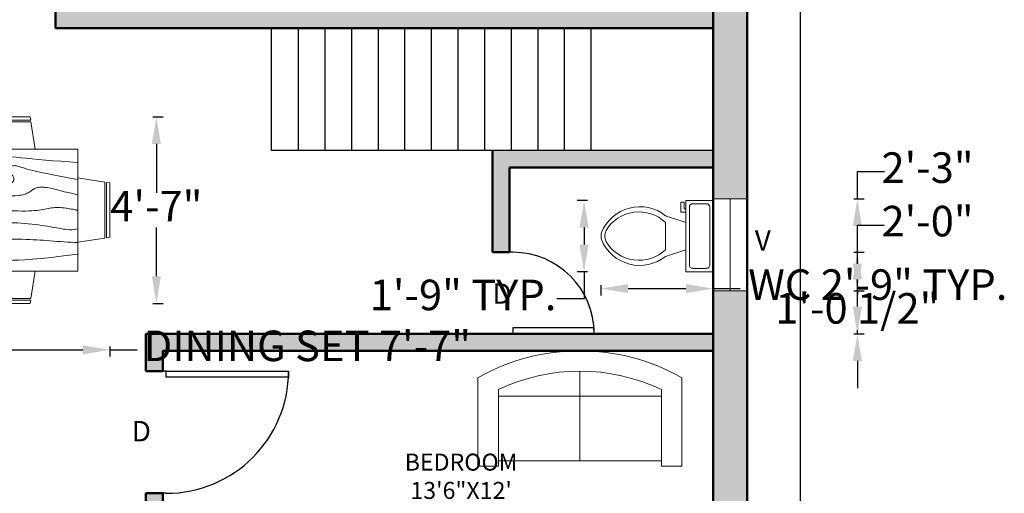
# Model space of a CAD drawing. Units: inches. Extents: x 2568 to 3190, y 746 to 1467.
# Tile 4 of 7: x 2900 to 3190, y 933 to 1073. Entities that reach past the tile are written whole.
import ezdxf

# ---------------------------------------------------------------- set-up
doc = ezdxf.new("R2010")
doc.units = ezdxf.units.IN
for name, color, linetype, lineweight in [('A-ANNO-DIMS', 2, 'Continuous', 18), ('A-ANNO-TEXT', 7, 'Continuous', 18), ('A-AREA-IDEN', 7, 'Continuous', 25), ('A-DOOR', 3, 'Continuous', 25), ('A-FLOR-FIXT', 9, 'Continuous', 20), ('A-FLOR-STRS', 7, 'Continuous', 25), ('A-FURN', 8, 'Continuous', 18), ('A-GLAZ', 4, 'Continuous', 20), ('A-WALL', 7, 'Continuous', 50), ('A-WALL-PATT', 252, 'Continuous', 13)]:
    doc.layers.add(name, color=color, linetype=linetype, lineweight=lineweight)
doc.styles.get("Standard").update_dxf_attribs({"font": 'arial.ttf'})
doc.dimstyles.new('ISO-25', dxfattribs={"dimtxt": 9, "dimasz": 8, "dimexe": 2, "dimexo": 1, "dimtad": 0, "dimtih": 1, "dimtoh": 1, "dimdec": 1, "dimlunit": 3, "dimtxsty": 'Standard', "dimcen": 2.5, "dimclrd": 1, "dimclre": 3, "dimclrt": 6, "dimadec": 0, "dimazin": 0, "dimtfac": 1, "dimtdec": 1, "dimtmove": 0, "dimatfit": 3, "dimfxl": 1, "dimfxlon": 1, "dimarcsym": 0})

# ---------------------------------------------------------------- blocks, each defined once
blk = doc.blocks.new('*U7')
for p, q in [((0, 0), (0, -6)), ((36, 0), (36, -6))]:
    blk.add_line(p, q)
blk.add_lwpolyline([(0, 0), (0, 36), (1.75, 36), (1.75, 0)], close=True)
blk.add_arc((0, 0), 36, 0, 90)
blk = doc.blocks.new('*U2')
for p, q in [((-24, 0), (-24, -6)), ((0, 0), (0, -6))]:
    blk.add_line(p, q)
blk.add_lwpolyline([(0, 0), (0, 24), (-1.75, 24), (-1.75, 0)], close=True)
blk.add_arc((0, 0), 24, 90, 180)
blk = doc.blocks.new('Dining Set - 36 x 72 in.')
for p, q in [((-22, 27.5), (-22.1562, 26.50042)), ((-5.8416, 26.5), (-22.1534, 26.5)), ((-22, 27.5), (-6, 27.5)), ((-5.8437, 26.49966), (-6, 27.5)), ((6, 27.5), (5.8438, 26.50042)), ((22.1584, 26.5), (5.8466, 26.5)), ((6, 27.5), (22, 27.5)), ((22.1563, 26.49966), (22, 27.5)), ((-22.2343, 26.00059), (-23.4847, 17.99762)), ((-22.2304, 26), (-5.7608, 26)), ((-4.5152, 17.99762), (-5.7655, 25.99926)), ((5.7657, 26.00059), (4.5153, 17.99762)), ((5.7696, 26), (22.2392, 26)), ((23.4848, 17.99762), (22.2345, 25.99926)), ((36, 18), (-36, 18)), ((-36, 18), (-36, -18)), ((36, -18), (36, 18)), ((-44.0006, 8.23428), (-35.9976, 9.48474)), ((44.0006, 8.23428), (35.9976, 9.48474)), ((-45.5, 8), (-44.5004, 8.15617)), ((-45.5, 8), (-45.5, -8)), ((-44.5, -8.15843), (-44.5, 8.15338)), ((-44, 8.23041), (-44, -8.23915)), ((44, 8.23041), (44, -8.23915)), ((44.5, -8.15843), (44.5, 8.15338)), ((45.5, 8), (44.5005, 8.15617)), ((45.5, 8), (45.5, -8)), ((-44.4997, -8.15631), (-45.5, -8)), ((-35.9976, -9.48476), (-43.9993, -8.2345)), ((35.9976, -9.48476), (43.9993, -8.2345)), ((44.4997, -8.15631), (45.5, -8)), ((-36, -18), (36, -18)), ((-22.2343, -26.0006), (-23.4847, -17.99762)), ((-4.5152, -17.99762), (-5.7655, -25.99928)), ((5.7657, -26.0006), (4.5153, -17.99762)), ((23.4848, -17.99762), (22.2345, -25.99928)), ((-22.2304, -26), (-5.7608, -26)), ((5.7696, -26), (22.2392, -26)), ((-22, -27.5), (-22.1562, -26.50044)), ((-5.8416, -26.5), (-22.1534, -26.5)), ((-22, -27.5), (-6, -27.5)), ((-5.8437, -26.49967), (-6, -27.5)), ((6, -27.5), (5.8438, -26.50044)), ((22.1584, -26.5), (5.8466, -26.5)), ((6, -27.5), (22, -27.5)), ((22.1563, -26.49967), (22, -27.5))]:
    blk.add_line(p, q)
for points in [[(-36, 15), (-31.1772, 14.97754), (-26.8079, 14.91406), (-22.8538, 14.81543), (-19.276, 14.6875), (-16.0362, 14.53613), (-13.0957, 14.36718), (-10.4159, 14.18652), (-7.9583, 14), (-5.6904, 13.81315), (-3.6035, 13.63021), (-1.6954, 13.45508), (0.0365, 13.29166), (1.5945, 13.14388), (2.9811, 13.01562), (4.1988, 12.9108), (5.25, 12.83333), (6.1393, 12.78613), (6.8802, 12.76823), (7.4883, 12.77767), (7.9792, 12.8125), (8.3685, 12.87077), (8.6719, 12.95052), (8.9049, 13.0498), (9.0833, 13.16666), (9.2205, 13.29899), (9.3216, 13.44401), (9.3895, 13.59879), (9.4271, 13.76041), (9.4373, 13.92594), (9.4232, 14.09245), (9.3875, 14.257), (9.3333, 14.41666), (9.2638, 14.56917), (9.1836, 14.71484), (9.0975, 14.85465), (9.0104, 14.98958), (8.9272, 15.1206), (8.8529, 15.2487), (8.7922, 15.37483), (8.75, 15.5), (8.7305, 15.62467), (8.7344, 15.74739), (8.7617, 15.86621), (8.8125, 15.97916), (8.8867, 16.08431), (8.9844, 16.17968), (9.1055, 16.26334), (9.25, 16.33333), (9.4189, 16.38802), (9.6172, 16.42708), (9.8506, 16.45052), (10.125, 16.45833), (10.4463, 16.45052), (10.8203, 16.42708), (11.2529, 16.38802), (11.75, 16.33333), (12.3184, 16.26318), (12.9694, 16.17838), (13.7151, 16.07991), (14.5677, 15.96875), (15.5395, 15.84586), (16.6426, 15.71224), (17.8893, 15.56884), (19.2917, 15.41666), (20.859, 15.25667), (22.5879, 15.08984), (24.4721, 14.91715), (26.5052, 14.73958), (28.6809, 14.5581), (30.9929, 14.3737), (33.4347, 14.18733), (36, 14)], [(-36, 10), (-28.9766, 10.14274), (-23.1725, 10.20442), (-18.4241, 10.19775), (-14.5677, 10.13541), (-11.4399, 10.03011), (-8.877, 9.89453), (-6.7154, 9.74137), (-4.7917, 9.58333), (-2.9698, 9.43082), (-1.2246, 9.28515), (0.4415, 9.14534), (2.026, 9.01041), (3.5266, 8.87939), (4.9408, 8.7513), (6.266, 8.62516), (7.5, 8.5), (8.6411, 8.37549), (9.6914, 8.2539), (10.6538, 8.13818), (11.5312, 8.03125), (12.3267, 7.93603), (13.043, 7.85547), (13.6831, 7.79248), (14.25, 7.75), (14.7471, 7.7303), (15.1797, 7.73307), (15.5537, 7.75732), (15.875, 7.80208), (16.1494, 7.86637), (16.3828, 7.94922), (16.5811, 8.04964), (16.75, 8.16666), (16.8944, 8.29915), (17.0143, 8.44531), (17.1089, 8.60319), (17.1771, 8.77083), (17.218, 8.94629), (17.2305, 9.1276), (17.2137, 9.31282), (17.1667, 9.5), (17.0895, 9.6875), (16.987, 9.875), (16.8649, 10.0625), (16.7292, 10.25), (16.5856, 10.4375), (16.4401, 10.625), (16.2985, 10.8125), (16.1667, 11), (16.05, 11.18733), (15.9518, 11.3737), (15.8752, 11.5581), (15.8229, 11.73958), (15.798, 11.91715), (15.8034, 12.08984), (15.842, 12.25667), (15.9167, 12.41666), (16.0295, 12.56836), (16.1784, 12.70833), (16.3605, 12.83268), (16.5729, 12.9375), (16.8127, 13.01888), (17.0768, 13.07291), (17.3625, 13.0957), (17.6667, 13.08333), (17.9894, 13.03312), (18.3418, 12.94726), (18.7382, 12.82918), (19.1927, 12.68229), (19.7195, 12.51001), (20.3327, 12.31575), (21.0465, 12.10294), (21.875, 11.875), (22.8357, 11.63354), (23.959, 11.37304), (25.2786, 11.08618), (26.8282, 10.76562), (28.6414, 10.40405), (30.752, 9.99414), (33.1936, 9.52856), (36, 9)], [(-36, 5.5), (-30.7157, 5.3348), (-26.069, 5.20963), (-21.9946, 5.11767), (-18.4271, 5.05208), (-15.3009, 5.00602), (-12.5508, 4.97265), (-10.1112, 4.94515), (-7.9167, 4.91666), (-5.909, 4.88167), (-4.0586, 4.83984), (-2.3429, 4.79215), (-0.7396, 4.73958), (0.7739, 4.6831), (2.22, 4.6237), (3.6213, 4.56233), (5, 4.5), (6.373, 4.43782), (7.7344, 4.3776), (9.0723, 4.32129), (10.375, 4.27083), (11.6309, 4.22819), (12.8281, 4.19531), (13.9551, 4.17415), (15, 4.16666), (15.954, 4.17448), (16.819, 4.19791), (17.6001, 4.23698), (18.3021, 4.29166), (18.9299, 4.36198), (19.4883, 4.44791), (19.9823, 4.54948), (20.4167, 4.66666), (20.7969, 4.79899), (21.1302, 4.94401), (21.4245, 5.09879), (21.6875, 5.26041), (21.9271, 5.42594), (22.1511, 5.59245), (22.3672, 5.757), (22.5834, 5.91666), (22.8065, 6.06868), (23.0404, 6.21093), (23.2879, 6.34147), (23.5521, 6.45833), (23.8358, 6.55957), (24.142, 6.64323), (24.4735, 6.70735), (24.8334, 6.75), (25.2235, 6.76969), (25.642, 6.76692), (26.0858, 6.74267), (26.5521, 6.69791), (27.0379, 6.63362), (27.5404, 6.55078), (28.0565, 6.45036), (28.5834, 6.33333), (29.1242, 6.19987), (29.7071, 6.04687), (30.3661, 5.87044), (31.1354, 5.66666), (32.0493, 5.43164), (33.142, 5.16146), (34.4475, 4.85221), (36, 4.5)], [(-36, -1), (-30.7915, -0.6591), (-26.0195, -0.38216), (-21.6519, -0.16284), (-17.6563, 0.00521), (-14.0005, 0.12833), (-10.6523, 0.21289), (-7.5796, 0.26522), (-4.75, 0.29166), (-2.134, 0.29793), (0.2878, 0.28711), (2.5317, 0.26163), (4.6146, 0.22396), (6.5529, 0.17651), (8.3633, 0.12174), (10.0623, 0.06209), (11.6667, 0), (13.1899, -0.06201), (14.6341, -0.1211), (15.9982, -0.17432), (17.2813, -0.21875), (18.4823, -0.25147), (19.6003, -0.26953), (20.6343, -0.27002), (21.5834, -0.25), (22.4481, -0.20768), (23.2357, -0.14584), (23.9549, -0.06836), (24.6146, 0.02083), (25.2235, 0.11784), (25.7904, 0.21875), (26.3241, 0.31966), (26.8334, 0.41666), (27.3265, 0.50618), (27.8099, 0.58593), (28.2894, 0.65397), (28.7709, 0.70833), (29.2601, 0.74707), (29.763, 0.76823), (30.2855, 0.76985), (30.8334, 0.75), (31.4088, 0.70784), (31.9994, 0.64713), (32.589, 0.57275), (33.1615, 0.48958), (33.7008, 0.4025), (34.1908, 0.3164), (34.6153, 0.23616), (34.9584, 0.16666), (35.2099, 0.11165), (35.3848, 0.07031), (35.504, 0.04069), (35.5886, 0.02083), (35.6594, 0.00879), (35.7377, 0.0026), (35.8442, 0.00032), (36, 0)], [(-36, -6.5), (-27.1843, -6.31267), (-20.084, -6.1263), (-14.469, -5.9419), (-10.1094, -5.76042), (-6.7752, -5.58285), (-4.2363, -5.41016), (-2.2629, -5.24333), (-0.625, -5.08334), (0.8708, -4.93099), (2.2715, -4.78646), (3.5872, -4.64974), (4.8281, -4.52084), (6.0046, -4.39974), (7.127, -4.28646), (8.2053, -4.18099), (9.25, -4.08334), (10.2705, -3.99382), (11.2734, -3.91407), (12.2647, -3.84603), (13.25, -3.79167), (14.2354, -3.75293), (15.2266, -3.73177), (16.2295, -3.73015), (17.25, -3.75), (18.2912, -3.79248), (19.3451, -3.85547), (20.4009, -3.93604), (21.4479, -4.03125), (22.4754, -4.13819), (23.4727, -4.25391), (24.4289, -4.37549), (25.3334, -4.5), (26.1785, -4.62492), (26.9694, -4.74935), (27.7145, -4.87281), (28.4219, -4.99479), (29.1, -5.11483), (29.7572, -5.23242), (30.4016, -5.34709), (31.0417, -5.45834), (31.6837, -5.56437), (32.3262, -5.65821), (32.9658, -5.73153), (33.599, -5.77604), (34.2224, -5.78345), (34.8327, -5.74545), (35.4264, -5.65373), (36, -5.5)], [(-36, -10), (-26.4022, -9.81299), (-18.4675, -9.62891), (-11.9839, -9.45069), (-6.7396, -9.28125), (-2.5226, -9.12354), (0.8789, -8.98047), (3.6769, -8.85498), (6.0833, -8.75), (8.2767, -8.66765), (10.3021, -8.60677), (12.1712, -8.56543), (13.8958, -8.54167), (15.4876, -8.53353), (16.9583, -8.53907), (18.3197, -8.55632), (19.5834, -8.58334), (20.7616, -8.61841), (21.8685, -8.66081), (22.9188, -8.71004), (23.9271, -8.76563), (24.9081, -8.82707), (25.8763, -8.89388), (26.8465, -8.96558), (27.8334, -9.04167), (28.8474, -9.12118), (29.8828, -9.20117), (30.93, -9.27824), (31.9792, -9.34896), (33.0205, -9.40991), (34.0443, -9.45768), (35.0407, -9.48885), (36, -9.5)], [(-36, -14.5), (-30.0881, -14.33513), (-25.0332, -14.21224), (-20.7312, -14.12647), (-17.0781, -14.07292), (-13.97, -14.04671), (-11.3027, -14.04297), (-8.9724, -14.05681), (-6.875, -14.08334), (-4.9224, -14.11833), (-3.0905, -14.16016), (-1.3709, -14.20785), (0.2448, -14.26042), (1.7647, -14.3169), (3.1973, -14.3763), (4.5507, -14.43767), (5.8333, -14.5), (7.0554, -14.5621), (8.235, -14.62175), (9.3922, -14.67652), (10.5469, -14.72396), (11.7192, -14.76164), (12.929, -14.78711), (14.1965, -14.79794), (15.5417, -14.79167), (16.9933, -14.76424), (18.6152, -14.70508), (20.4804, -14.60197), (22.6615, -14.44271), (25.2312, -14.21509), (28.2624, -13.9069), (31.8277, -13.50594), (36, -13)]]:
    blk.add_lwpolyline(points)
blk = doc.blocks.new('Toilet - top')
for p, q in [((9.5, -6), (9.5, -2)), ((-10, -8.5), (-8, -8.5)), ((-10, -9.5), (-10, -8.5)), ((-8, -8.5), (-8, -8)), ((-7, -8), (-7, -9.5)), ((-4, -8), (-6, -14)), ((4, -8), (6, -14)), ((-7, -9.5), (-10, -9.5)), ((4, -14), (-4, -14))]:
    blk.add_line(p, q)
blk.add_lwpolyline([(10.5, -8), (10.5, 0), (-10.5, 0), (-10.5, -8)], close=True)
for points in [[(-9.5, -2), (-9.5, -6)], [(8.5, -1), (-8.5, -1)], [(-8.5, -7), (8.5, -7)]]:
    blk.add_lwpolyline(points)
for centre, radius, start, end in [((-8.62, -1.88), 0.884, 81.8699, 188.1301), ((8.62, -1.88), 0.884, 351.8699, 98.1301), ((-8.62, -6.12), 0.884, 171.8699, 278.1301), ((8.62, -6.12), 0.884, 261.8699, 8.1301), ((3.52, -21.58), 12.17, 141.4691, 247.9714), ((4.2, -21.82), 11.33, 136.3677, 238.9468), ((-3.52, -21.58), 12.17, 292.0284, 38.5307), ((-4.2, -21.82), 11.33, 301.053, 43.6321), ((0, -27.88), 4, 245.7318, 294.2682), ((0, -29), 4, 254.8605, 285.1395)]:
    blk.add_arc(centre, radius, start, end)
blk = doc.blocks.new('*D14')
at = {"layer": 'A-ANNO-DIMS', "color": 0, "lineweight": -2, "transparency": 16777216}
for p, q in [((3129.28, 1421.35), (3132.28, 1421.35)), ((3130.28, 1413.35), (3130.28, 1126.57)), ((3130.28, 829.35), (3130.28, 1116.13)), ((3129.28, 821.35), (3132.28, 821.35))]:
    blk.add_line(p, q, dxfattribs=at)
at = {"layer": 'A-ANNO-DIMS', "color": 0, "transparency": 16777216}
for points in [[(3128.95, 1413.35), (3131.61, 1413.35), (3130.28, 1421.35)], [(3128.95, 829.35), (3131.61, 829.35), (3130.28, 821.35)]]:
    blk.add_solid(points, dxfattribs=at)
at = {"layer": 'Defpoints', "color": 0, "transparency": 16777216}
for p in [(3114.52, 1421.35), (3114.52, 821.35), (3130.28, 821.35)]:
    blk.add_point(p, dxfattribs=at)
at = {"layer": 'A-ANNO-DIMS', "color": 0, "transparency": 16777216, "insert": (3130.28, 1121.35), "char_height": 9, "attachment_point": 5}
blk.add_mtext("50'", dxfattribs=at)
blk = doc.blocks.new('Sofa - Roundback Loveseat 5 ft.')
for p, q in [((0, -32.44198), (0, -5.99998)), ((-24, -33.99998), (-24, -11.46958)), ((24.00004, -33.99998), (24.00004, -11.46958)), ((-23.9998, -13.38178), (23.99986, -13.38178)), ((-24, -32.44198), (24.00004, -32.44198))]:
    blk.add_line(p, q)
for points in [[(-24, -33.99998), (-30, -33.99998), (-30, -7.99998)], [(30.00004, -7.99998), (30.00004, -33.99998), (24.00004, -33.99998)]]:
    blk.add_lwpolyline(points)
for centre, radius, start, end in [((0, -60.24998), 60.24998, 60.13715, 119.8628), ((0, -61.38438), 55.38444, 64.32083, 115.6792)]:
    blk.add_arc(centre, radius, start, end)
blk = doc.blocks.new('*D27')
at = {"layer": 'A-ANNO-DIMS', "color": 3, "lineweight": -2, "transparency": 16777216}
for p, q in [((3071.48, 994.65), (3071.48, 991.65)), ((3104.52, 994.65), (3104.52, 991.65))]:
    blk.add_line(p, q, dxfattribs=at)
at = {"layer": 'A-ANNO-DIMS', "color": 1, "lineweight": -2, "transparency": 16777216}
for p, q in [((3079.48, 993.65), (3096.52, 993.65)), ((3104.52, 993.65), (3112.52, 993.65))]:
    blk.add_line(p, q, dxfattribs=at)
at = {"layer": 'A-ANNO-DIMS', "color": 1, "transparency": 16777216}
for points in [[(3079.48, 994.99), (3079.48, 992.32), (3071.48, 993.65)], [(3096.52, 994.99), (3096.52, 992.32), (3104.52, 993.65)]]:
    blk.add_solid(points, dxfattribs=at)
at = {"layer": 'Defpoints', "color": 0, "transparency": 16777216}
for p in [(3071.48, 998.61), (3104.52, 998.61), (3104.52, 993.65)]:
    blk.add_point(p, dxfattribs=at)
at = {"layer": 'A-ANNO-DIMS', "color": 6, "transparency": 16777216, "insert": (3152.98, 993.65), "char_height": 9, "attachment_point": 5}
blk.add_mtext('WC 2\'-9" TYP.', dxfattribs=at)
blk = doc.blocks.new('*D28')
at = {"layer": 'A-ANNO-DIMS', "color": 3, "lineweight": -2, "transparency": 16777216}
for p, q in [((3067.52, 1019.61), (3064.52, 1019.61)), ((3067.52, 998.61), (3064.52, 998.61))]:
    blk.add_line(p, q, dxfattribs=at)
at = {"layer": 'A-ANNO-DIMS', "color": 1, "lineweight": -2, "transparency": 16777216}
for p, q in [((3066.52, 1011.61), (3066.52, 1006.61)), ((3066.52, 998.61), (3066.52, 990.61)), ((3066.52, 990.61), (3058.52, 990.61))]:
    blk.add_line(p, q, dxfattribs=at)
at = {"layer": 'A-ANNO-DIMS', "color": 1, "transparency": 16777216}
for points in [[(3065.19, 1011.61), (3067.85, 1011.61), (3066.52, 1019.61)], [(3065.19, 1006.61), (3067.85, 1006.61), (3066.52, 998.61)]]:
    blk.add_solid(points, dxfattribs=at)
at = {"layer": 'Defpoints', "color": 0, "transparency": 16777216}
for p in [(3071.48, 1019.61), (3066.52, 998.61), (3071.48, 998.61)]:
    blk.add_point(p, dxfattribs=at)
at = {"layer": 'A-ANNO-DIMS', "color": 6, "transparency": 16777216, "insert": (3030.89, 990.61), "char_height": 9, "attachment_point": 5}
blk.add_mtext('1\'-9" TYP.', dxfattribs=at)
blk = doc.blocks.new('*D37')
at = {"layer": 'A-ANNO-DIMS', "color": 3, "lineweight": -2, "transparency": 16777216}
for p, q in [((2835.95, 976.61), (2835.95, 973.61)), ((2926.95, 976.61), (2926.95, 973.61))]:
    blk.add_line(p, q, dxfattribs=at)
at = {"layer": 'A-ANNO-DIMS', "color": 1, "lineweight": -2, "transparency": 16777216}
for p, q in [((2843.95, 975.61), (2918.95, 975.61)), ((2926.95, 975.61), (2934.95, 975.61))]:
    blk.add_line(p, q, dxfattribs=at)
at = {"layer": 'A-ANNO-DIMS', "color": 1, "transparency": 16777216}
for points in [[(2843.95, 976.94), (2843.95, 974.27), (2835.95, 975.61)], [(2918.95, 976.94), (2918.95, 974.27), (2926.95, 975.61)]]:
    blk.add_solid(points, dxfattribs=at)
at = {"layer": 'Defpoints', "color": 0, "transparency": 16777216}
for p in [(2835.95, 989.26), (2926.95, 989.26), (2926.95, 975.61)]:
    blk.add_point(p, dxfattribs=at)
at = {"layer": 'A-ANNO-DIMS', "color": 6, "transparency": 16777216, "insert": (2985.04, 975.61), "char_height": 9, "attachment_point": 5}
blk.add_mtext('DINING SET 7\'-7"', dxfattribs=at)
blk = doc.blocks.new('*D38')
at = {"layer": 'A-ANNO-DIMS', "color": 3, "lineweight": -2, "transparency": 16777216}
for p, q in [((2939.6, 1044.26), (2942.6, 1044.26)), ((2939.6, 989.26), (2942.6, 989.26))]:
    blk.add_line(p, q, dxfattribs=at)
at = {"layer": 'A-ANNO-DIMS', "color": 1, "lineweight": -2, "transparency": 16777216}
for p, q in [((2940.6, 1036.26), (2940.6, 1021.88)), ((2940.6, 997.26), (2940.6, 1011.63))]:
    blk.add_line(p, q, dxfattribs=at)
at = {"layer": 'A-ANNO-DIMS', "color": 1, "transparency": 16777216}
for points in [[(2939.27, 1036.26), (2941.94, 1036.26), (2940.6, 1044.26)], [(2939.27, 997.26), (2941.94, 997.26), (2940.6, 989.26)]]:
    blk.add_solid(points, dxfattribs=at)
at = {"layer": 'Defpoints', "color": 0, "transparency": 16777216}
for p in [(2926.95, 1044.26), (2940.6, 1044.26), (2926.95, 989.26)]:
    blk.add_point(p, dxfattribs=at)
at = {"layer": 'A-ANNO-DIMS', "color": 6, "transparency": 16777216, "insert": (2940.6, 1016.76), "char_height": 9, "attachment_point": 5}
blk.add_mtext('4\'-7"', dxfattribs=at)
blk = doc.blocks.new('*D43')
at = {"layer": 'A-ANNO-DIMS', "color": 1, "lineweight": -2, "transparency": 16777216}
for p, q in [((2934.52, 759.85), (2926.52, 759.85)), ((2942.52, 759.85), (2946.11, 759.85)), ((2996.2, 759.85), (2992.62, 759.85)), ((3004.2, 759.85), (3012.2, 759.85))]:
    blk.add_line(p, q, dxfattribs=at)
at = {"layer": 'A-ANNO-DIMS', "color": 3, "lineweight": -2, "transparency": 16777216}
for p, q in [((2942.52, 760.85), (2942.52, 757.85)), ((2996.2, 760.85), (2996.2, 757.85))]:
    blk.add_line(p, q, dxfattribs=at)
at = {"layer": 'A-ANNO-DIMS', "color": 1, "transparency": 16777216}
for points in [[(2934.52, 761.18), (2934.52, 758.51), (2942.52, 759.85)], [(3004.2, 761.18), (3004.2, 758.51), (2996.2, 759.85)]]:
    blk.add_solid(points, dxfattribs=at)
at = {"layer": 'Defpoints', "color": 0, "transparency": 16777216}
for p in [(2942.52, 1411.35), (2996.2, 1411.35), (2996.2, 759.85)]:
    blk.add_point(p, dxfattribs=at)
at = {"layer": 'A-ANNO-DIMS', "color": 6, "transparency": 16777216, "insert": (2969.36, 759.85), "char_height": 9, "attachment_point": 5}
blk.add_mtext('4\'-5 1/2"', dxfattribs=at)
blk = doc.blocks.new('*D44')
at = {"layer": 'A-ANNO-DIMS', "color": 1, "lineweight": -2, "transparency": 16777216}
for p, q in [((2988.2, 759.85), (2980.2, 759.85)), ((2996.2, 759.85), (3001.17, 759.85)), ((3052.64, 759.85), (3047.67, 759.85)), ((3060.64, 759.85), (3068.64, 759.85))]:
    blk.add_line(p, q, dxfattribs=at)
at = {"layer": 'A-ANNO-DIMS', "color": 3, "lineweight": -2, "transparency": 16777216}
for p, q in [((2996.2, 760.85), (2996.2, 757.85)), ((3052.64, 760.85), (3052.64, 757.85))]:
    blk.add_line(p, q, dxfattribs=at)
at = {"layer": 'A-ANNO-DIMS', "color": 1, "transparency": 16777216}
for points in [[(2988.2, 761.18), (2988.2, 758.51), (2996.2, 759.85)], [(3060.64, 761.18), (3060.64, 758.51), (3052.64, 759.85)]]:
    blk.add_solid(points, dxfattribs=at)
at = {"layer": 'Defpoints', "color": 0, "transparency": 16777216}
for p in [(2996.2, 1411.35), (3052.64, 1411.35), (3052.64, 759.85)]:
    blk.add_point(p, dxfattribs=at)
at = {"layer": 'A-ANNO-DIMS', "color": 6, "transparency": 16777216, "insert": (3024.42, 759.85), "char_height": 9, "attachment_point": 5}
blk.add_mtext('4\'-8 1/2"', dxfattribs=at)
blk = doc.blocks.new('*D50')
at = {"layer": 'A-ANNO-DIMS', "color": 3, "lineweight": -2, "transparency": 16777216}
for p, q in [((2846.86, 1452.8), (2846.86, 1455.8)), ((2902.21, 1452.8), (2902.21, 1455.8))]:
    blk.add_line(p, q, dxfattribs=at)
at = {"layer": 'A-ANNO-DIMS', "color": 1, "lineweight": -2, "transparency": 16777216}
for p, q in [((2838.86, 1453.8), (2830.86, 1453.8)), ((2846.86, 1453.8), (2851.29, 1453.8)), ((2902.21, 1453.8), (2897.79, 1453.8)), ((2910.21, 1453.8), (2918.21, 1453.8))]:
    blk.add_line(p, q, dxfattribs=at)
at = {"layer": 'A-ANNO-DIMS', "color": 1, "transparency": 16777216}
for points in [[(2838.86, 1455.13), (2838.86, 1452.47), (2846.86, 1453.8)], [(2910.21, 1455.13), (2910.21, 1452.47), (2902.21, 1453.8)]]:
    blk.add_solid(points, dxfattribs=at)
at = {"layer": 'Defpoints', "color": 0, "transparency": 16777216}
for p in [(2902.21, 1453.8), (2846.86, 831.35), (2902.21, 831.35)]:
    blk.add_point(p, dxfattribs=at)
at = {"layer": 'A-ANNO-DIMS', "color": 6, "transparency": 16777216, "insert": (2874.54, 1453.8), "char_height": 9, "attachment_point": 5}
blk.add_mtext('4\'-7 1/2"', dxfattribs=at)
blk = doc.blocks.new('*D56')
at = {"layer": 'A-ANNO-DIMS', "color": 3, "lineweight": -2, "transparency": 16777216}
for p, q in [((2603.07, 1070.35), (2600.07, 1070.35)), ((2603.07, 1034.35), (2600.07, 1034.35))]:
    blk.add_line(p, q, dxfattribs=at)
at = {"layer": 'A-ANNO-DIMS', "color": 1, "lineweight": -2, "transparency": 16777216}
for p, q in [((2602.07, 1062.35), (2602.07, 1057.57)), ((2602.07, 1042.35), (2602.07, 1047.13))]:
    blk.add_line(p, q, dxfattribs=at)
at = {"layer": 'A-ANNO-DIMS', "color": 1, "transparency": 16777216}
for points in [[(2600.74, 1062.35), (2603.41, 1062.35), (2602.07, 1070.35)], [(2600.74, 1042.35), (2603.41, 1042.35), (2602.07, 1034.35)]]:
    blk.add_solid(points, dxfattribs=at)
at = {"layer": 'Defpoints', "color": 0, "transparency": 16777216}
for p in [(2602.07, 1070.35), (2974.52, 1070.35), (2974.52, 1034.35)]:
    blk.add_point(p, dxfattribs=at)
at = {"layer": 'A-ANNO-DIMS', "color": 6, "transparency": 16777216, "insert": (2602.07, 1052.35), "char_height": 9, "attachment_point": 5}
blk.add_mtext('3\'-0"', dxfattribs=at)
blk = doc.blocks.new('*D57')
at = {"layer": 'A-ANNO-DIMS', "color": 3, "lineweight": -2, "transparency": 16777216}
for p, q in [((2974.52, 1452.8), (2974.52, 1455.8)), ((3104.52, 1452.8), (3104.52, 1455.8))]:
    blk.add_line(p, q, dxfattribs=at)
at = {"layer": 'A-ANNO-DIMS', "color": 1, "lineweight": -2, "transparency": 16777216}
for p, q in [((2982.52, 1453.8), (3020.37, 1453.8)), ((3096.52, 1453.8), (3058.68, 1453.8))]:
    blk.add_line(p, q, dxfattribs=at)
at = {"layer": 'A-ANNO-DIMS', "color": 1, "transparency": 16777216}
for points in [[(2982.52, 1455.13), (2982.52, 1452.47), (2974.52, 1453.8)], [(3096.52, 1455.13), (3096.52, 1452.47), (3104.52, 1453.8)]]:
    blk.add_solid(points, dxfattribs=at)
at = {"layer": 'Defpoints', "color": 0, "transparency": 16777216}
for p in [(3104.52, 1453.8), (2974.52, 1070.35), (3104.52, 1070.35)]:
    blk.add_point(p, dxfattribs=at)
at = {"layer": 'A-ANNO-DIMS', "color": 6, "transparency": 16777216, "insert": (3039.52, 1453.8), "char_height": 9, "attachment_point": 5}
blk.add_mtext('10\'-10"', dxfattribs=at)
blk = doc.blocks.new('*D58')
at = {"layer": 'A-ANNO-DIMS', "color": 3, "lineweight": -2, "transparency": 16777216}
for p, q in [((2603.07, 1029.35), (2600.07, 1029.35)), ((2603.07, 980.35), (2600.07, 980.35))]:
    blk.add_line(p, q, dxfattribs=at)
at = {"layer": 'A-ANNO-DIMS', "color": 1, "lineweight": -2, "transparency": 16777216}
for p, q in [((2602.07, 1021.35), (2602.07, 1009.99)), ((2602.07, 988.35), (2602.07, 999.71))]:
    blk.add_line(p, q, dxfattribs=at)
at = {"layer": 'A-ANNO-DIMS', "color": 1, "transparency": 16777216}
for points in [[(2600.74, 1021.35), (2603.41, 1021.35), (2602.07, 1029.35)], [(2600.74, 988.35), (2603.41, 988.35), (2602.07, 980.35)]]:
    blk.add_solid(points, dxfattribs=at)
at = {"layer": 'Defpoints', "color": 0, "transparency": 16777216}
for p in [(3044.52, 1029.35), (2602.07, 980.35), (3043.77, 980.35)]:
    blk.add_point(p, dxfattribs=at)
at = {"layer": 'A-ANNO-DIMS', "color": 6, "transparency": 16777216, "insert": (2602.07, 1004.85), "char_height": 9, "attachment_point": 5}
blk.add_mtext('4\'-1"', dxfattribs=at)
blk = doc.blocks.new('*D59')
at = {"layer": 'A-ANNO-DIMS', "color": 3, "lineweight": -2, "transparency": 16777216}
for p, q in [((3044.52, 760.85), (3044.52, 757.85)), ((3104.52, 760.85), (3104.52, 757.85))]:
    blk.add_line(p, q, dxfattribs=at)
at = {"layer": 'A-ANNO-DIMS', "color": 1, "lineweight": -2, "transparency": 16777216}
for p, q in [((3052.52, 759.85), (3061.94, 759.85)), ((3096.52, 759.85), (3087.11, 759.85))]:
    blk.add_line(p, q, dxfattribs=at)
at = {"layer": 'A-ANNO-DIMS', "color": 1, "transparency": 16777216}
for points in [[(3052.52, 761.18), (3052.52, 758.51), (3044.52, 759.85)], [(3096.52, 761.18), (3096.52, 758.51), (3104.52, 759.85)]]:
    blk.add_solid(points, dxfattribs=at)
at = {"layer": 'Defpoints', "color": 0, "transparency": 16777216}
for p in [(3044.52, 1029.35), (3104.52, 1029.35), (3104.52, 759.85)]:
    blk.add_point(p, dxfattribs=at)
at = {"layer": 'A-ANNO-DIMS', "color": 6, "transparency": 16777216, "insert": (3074.52, 759.85), "char_height": 9, "attachment_point": 5}
blk.add_mtext('5\'-0"', dxfattribs=at)
blk = doc.blocks.new('*D60')
at = {"layer": 'A-ANNO-DIMS', "color": 1, "lineweight": -2, "transparency": 16777216}
for p, q in [((2966.52, 759.85), (2958.52, 759.85)), ((2974.52, 759.85), (2982.36, 759.85)), ((2990.36, 759.85), (2998.36, 759.85))]:
    blk.add_line(p, q, dxfattribs=at)
at = {"layer": 'A-ANNO-DIMS', "color": 3, "lineweight": -2, "transparency": 16777216}
for p, q in [((2974.52, 760.85), (2974.52, 757.85)), ((2982.36, 760.85), (2982.36, 757.85))]:
    blk.add_line(p, q, dxfattribs=at)
at = {"layer": 'A-ANNO-DIMS', "color": 1, "transparency": 16777216}
for points in [[(2966.52, 761.18), (2966.52, 758.51), (2974.52, 759.85)], [(2990.36, 761.18), (2990.36, 758.51), (2982.36, 759.85)]]:
    blk.add_solid(points, dxfattribs=at)
at = {"layer": 'Defpoints', "color": 0, "transparency": 16777216}
for p in [(2974.52, 1034.35), (2982.36, 1034.35), (2982.36, 759.85)]:
    blk.add_point(p, dxfattribs=at)
at = {"layer": 'A-ANNO-DIMS', "color": 6, "transparency": 16777216, "insert": (3010.94, 759.85), "char_height": 9, "attachment_point": 5}
blk.add_mtext('0\'-8"', dxfattribs=at)
blk = doc.blocks.new('*D61')
at = {"layer": 'A-ANNO-DIMS', "color": 3, "lineweight": -2, "transparency": 16777216}
for p, q in [((3068.52, 1452.8), (3068.52, 1455.8)), ((3104.52, 1452.8), (3104.52, 1455.8))]:
    blk.add_line(p, q, dxfattribs=at)
at = {"layer": 'A-ANNO-DIMS', "color": 1, "lineweight": -2, "transparency": 16777216}
for p, q in [((3060.52, 1453.8), (3052.52, 1453.8)), ((3068.52, 1453.8), (3073.94, 1453.8)), ((3104.52, 1453.8), (3099.11, 1453.8)), ((3112.52, 1453.8), (3120.52, 1453.8))]:
    blk.add_line(p, q, dxfattribs=at)
at = {"layer": 'A-ANNO-DIMS', "color": 1, "transparency": 16777216}
for points in [[(3060.52, 1455.13), (3060.52, 1452.47), (3068.52, 1453.8)], [(3112.52, 1455.13), (3112.52, 1452.47), (3104.52, 1453.8)]]:
    blk.add_solid(points, dxfattribs=at)
at = {"layer": 'Defpoints', "color": 0, "transparency": 16777216}
for p in [(3104.52, 1453.8), (3068.52, 1034.35), (3104.52, 1034.35)]:
    blk.add_point(p, dxfattribs=at)
at = {"layer": 'A-ANNO-DIMS', "color": 6, "transparency": 16777216, "insert": (3086.52, 1453.8), "char_height": 9, "attachment_point": 5}
blk.add_mtext('3\'-0"', dxfattribs=at)
blk = doc.blocks.new('*D62')
at = {"layer": 'A-ANNO-DIMS', "color": 3, "lineweight": -2, "transparency": 16777216}
for p, q in [((2603.07, 1004.35), (2600.07, 1004.35)), ((2603.07, 980.35), (2600.07, 980.35))]:
    blk.add_line(p, q, dxfattribs=at)
at = {"layer": 'A-ANNO-DIMS', "color": 1, "lineweight": -2, "transparency": 16777216}
for p, q in [((2602.07, 996.35), (2602.07, 988.35)), ((2602.07, 980.35), (2602.07, 972.35)), ((2602.07, 972.35), (2594.07, 972.35))]:
    blk.add_line(p, q, dxfattribs=at)
at = {"layer": 'A-ANNO-DIMS', "color": 1, "transparency": 16777216}
for points in [[(2600.74, 996.35), (2603.41, 996.35), (2602.07, 1004.35)], [(2600.74, 988.35), (2603.41, 988.35), (2602.07, 980.35)]]:
    blk.add_solid(points, dxfattribs=at)
at = {"layer": 'Defpoints', "color": 0, "transparency": 16777216}
for p in [(3044.52, 1004.35), (2602.07, 980.35), (3043.77, 980.35)]:
    blk.add_point(p, dxfattribs=at)
at = {"layer": 'A-ANNO-DIMS', "color": 6, "transparency": 16777216, "insert": (2581.41, 972.35), "char_height": 9, "attachment_point": 5}
blk.add_mtext('2\'-0"', dxfattribs=at)
blk = doc.blocks.new('*D63')
at = {"layer": 'A-ANNO-DIMS', "color": 1, "lineweight": -2, "transparency": 16777216}
for p, q in [((3146.97, 1004.35), (3146.97, 1012.35)), ((3146.97, 1012.35), (3154.97, 1012.35)), ((3146.97, 988.35), (3146.97, 996.35))]:
    blk.add_line(p, q, dxfattribs=at)
at = {"layer": 'A-ANNO-DIMS', "color": 3, "lineweight": -2, "transparency": 16777216}
for p, q in [((3145.97, 1004.35), (3148.97, 1004.35)), ((3145.97, 980.35), (3148.97, 980.35))]:
    blk.add_line(p, q, dxfattribs=at)
at = {"layer": 'A-ANNO-DIMS', "color": 1, "transparency": 16777216}
for points in [[(3145.64, 996.35), (3148.31, 996.35), (3146.97, 1004.35)], [(3145.64, 988.35), (3148.31, 988.35), (3146.97, 980.35)]]:
    blk.add_solid(points, dxfattribs=at)
at = {"layer": 'Defpoints', "color": 0, "transparency": 16777216}
for p in [(2806.52, 1004.35), (3146.97, 1004.35), (2806.52, 980.35)]:
    blk.add_point(p, dxfattribs=at)
at = {"layer": 'A-ANNO-DIMS', "color": 6, "transparency": 16777216, "insert": (3167.64, 1012.35), "char_height": 9, "attachment_point": 5}
blk.add_mtext('2\'-0"', dxfattribs=at)
blk = doc.blocks.new('*D72')
at = {"layer": 'A-ANNO-DIMS', "color": 1, "lineweight": -2, "transparency": 16777216}
for p, q in [((3146.97, 1020.11), (3146.97, 1028.11)), ((3146.97, 1028.11), (3154.97, 1028.11)), ((3146.97, 1000.96), (3146.97, 1012.11))]:
    blk.add_line(p, q, dxfattribs=at)
at = {"layer": 'A-ANNO-DIMS', "color": 3, "lineweight": -2, "transparency": 16777216}
for p, q in [((3145.97, 1020.11), (3148.97, 1020.11)), ((3145.97, 992.96), (3148.97, 992.96))]:
    blk.add_line(p, q, dxfattribs=at)
at = {"layer": 'A-ANNO-DIMS', "color": 1, "transparency": 16777216}
for points in [[(3145.64, 1012.11), (3148.31, 1012.11), (3146.97, 1020.11)], [(3145.64, 1000.96), (3148.31, 1000.96), (3146.97, 992.96)]]:
    blk.add_solid(points, dxfattribs=at)
at = {"layer": 'Defpoints', "color": 0, "transparency": 16777216}
for p in [(3114.52, 1020.11), (3146.97, 1020.11), (3114.52, 992.96)]:
    blk.add_point(p, dxfattribs=at)
at = {"layer": 'A-ANNO-DIMS', "color": 6, "transparency": 16777216, "insert": (3167.64, 1028.11), "char_height": 9, "attachment_point": 5}
blk.add_mtext('2\'-3"', dxfattribs=at)
blk = doc.blocks.new('*D73')
at = {"layer": 'A-ANNO-DIMS', "color": 1, "lineweight": -2, "transparency": 16777216}
for p, q in [((3146.97, 1000.96), (3146.97, 1008.96)), ((3146.97, 992.96), (3146.97, 991.93)), ((3146.97, 980.35), (3146.97, 981.38)), ((3146.97, 972.35), (3146.97, 964.35))]:
    blk.add_line(p, q, dxfattribs=at)
at = {"layer": 'A-ANNO-DIMS', "color": 3, "lineweight": -2, "transparency": 16777216}
for p, q in [((3145.97, 992.96), (3148.97, 992.96)), ((3145.97, 980.35), (3148.97, 980.35))]:
    blk.add_line(p, q, dxfattribs=at)
at = {"layer": 'A-ANNO-DIMS', "color": 1, "transparency": 16777216}
for points in [[(3145.64, 1000.96), (3148.31, 1000.96), (3146.97, 992.96)], [(3145.64, 972.35), (3148.31, 972.35), (3146.97, 980.35)]]:
    blk.add_solid(points, dxfattribs=at)
at = {"layer": 'Defpoints', "color": 0, "transparency": 16777216}
for p in [(3104.52, 992.96), (3146.97, 992.96), (3104.52, 980.35)]:
    blk.add_point(p, dxfattribs=at)
at = {"layer": 'A-ANNO-DIMS', "color": 6, "transparency": 16777216, "insert": (3146.97, 986.66), "char_height": 9, "attachment_point": 5}
blk.add_mtext('1\'-0 1/2"', dxfattribs=at)
blk = doc.blocks.new('*D76')
at = {"layer": 'A-ANNO-DIMS', "color": 3, "lineweight": -2, "transparency": 16777216}
for p, q in [((3044.52, 760.85), (3044.52, 757.85)), ((3104.52, 760.85), (3104.52, 757.85))]:
    blk.add_line(p, q, dxfattribs=at)
at = {"layer": 'A-ANNO-DIMS', "color": 1, "lineweight": -2, "transparency": 16777216}
for p, q in [((3052.52, 759.85), (3061.94, 759.85)), ((3096.52, 759.85), (3087.11, 759.85))]:
    blk.add_line(p, q, dxfattribs=at)
at = {"layer": 'A-ANNO-DIMS', "color": 1, "transparency": 16777216}
for points in [[(3052.52, 761.18), (3052.52, 758.51), (3044.52, 759.85)], [(3096.52, 761.18), (3096.52, 758.51), (3104.52, 759.85)]]:
    blk.add_solid(points, dxfattribs=at)
at = {"layer": 'Defpoints', "color": 0, "transparency": 16777216}
for p in [(3044.52, 1202.35), (3104.52, 1202.35), (3104.52, 759.85)]:
    blk.add_point(p, dxfattribs=at)
at = {"layer": 'A-ANNO-DIMS', "color": 6, "transparency": 16777216, "insert": (3074.52, 759.85), "char_height": 9, "attachment_point": 5}
blk.add_mtext('5\'-0"', dxfattribs=at)

msp = doc.modelspace()

# ---------------------------------------------------------------- hatches: boundary and pattern name
at = {"layer": 'A-WALL-PATT'}
h = msp.add_hatch(color=256, dxfattribs=at)
h.dxf.hatch_style = 1
h.paths.add_polyline_path([(2709.74, 1411.35), (2709.74, 1421.35), (2634.52, 1421.35), (2634.52, 1371.08), (2644.52, 1371.08), (2644.52, 1411.35)])
h.paths.add_polyline_path([(2844.66, 1411.35), (2844.66, 1421.35), (2763.78, 1421.35), (2763.78, 1411.35)])
h.paths.add_polyline_path([(2996.2, 1411.35), (2996.2, 1421.35), (2897.43, 1421.35), (2897.43, 1411.35)])
h.paths.add_polyline_path([(3104.52, 1411.35), (3104.52, 1371.08), (3114.52, 1371.08), (3114.52, 1421.35), (3052.64, 1421.35), (3052.64, 1411.35)])
h.paths.add_polyline_path([(3114.52, 1316.62), (3104.52, 1316.62), (3104.52, 1248.37), (3114.52, 1248.37)])
h.paths.add_polyline_path([(3104.52, 1174.04), (3114.52, 1174.04), (3114.52, 1222.08), (3104.52, 1222.08)])
h.paths.add_polyline_path([(3104.52, 1020.11), (3114.52, 1020.11), (3114.52, 1113), (3104.52, 1113)])
h.paths.add_polyline_path([(3104.52, 920.42), (3114.52, 920.42), (3114.52, 992.96), (3104.52, 992.96)])
h.paths.add_polyline_path([(3114.52, 821.35), (3114.52, 865.93), (3104.52, 865.93), (3104.52, 831.35), (3055.78, 831.35), (3055.78, 821.35)])
h.paths.add_polyline_path([(2902.21, 831.35), (2902.21, 821.35), (2986.63, 821.35), (2986.63, 831.35)])
h.paths.add_polyline_path([(2634.52, 821.35), (2676.76, 821.35), (2676.76, 831.35), (2644.52, 831.35), (2644.52, 865.93), (2634.52, 865.93)])
h.paths.add_polyline_path([(2754.37, 821.35), (2846.86, 821.35), (2846.86, 831.35), (2754.37, 831.35)])
h.paths.add_polyline_path([(2644.52, 920.42), (2644.52, 1002.57), (2634.52, 1002.57), (2634.52, 920.42)])
h.paths.add_polyline_path([(2644.52, 1044.16), (2644.52, 1113), (2634.52, 1113), (2634.52, 1044.16)])
h.paths.add_polyline_path([(2644.52, 1248.37), (2644.52, 1316.62), (2634.52, 1316.62), (2634.52, 1248.37)])
h.paths.add_polyline_path([(2634.52, 1222.08), (2634.52, 1174.04), (2644.52, 1174.04), (2644.52, 1222.08)])
h = msp.add_hatch(color=256, dxfattribs=at)
h.dxf.hatch_style = 1
h.paths.add_polyline_path([(2811.52, 1411.35), (2806.52, 1411.35), (2806.52, 1303.35), (2811.52, 1303.35), (2811.52, 1310.35), (2850.52, 1310.35), (2850.52, 1315.35), (2811.52, 1315.35)])
h.paths.add_polyline_path([(2942.52, 1411.35), (2937.52, 1411.35), (2937.52, 1315.35), (2898.52, 1315.35), (2898.52, 1310.35), (2937.52, 1310.35), (2937.52, 1303.35), (2942.52, 1303.35)])
h.paths.add_polyline_path([(2811.52, 1267.35), (2704.52, 1267.35), (2704.52, 1261.35), (2704.52, 1237.35), (2704.52, 1202.35), (2644.52, 1202.35), (2644.52, 1197.35), (2806.52, 1197.35), (2806.52, 1191.38), (2811.52, 1191.38), (2811.52, 1202.35), (2793.52, 1202.35), (2793.52, 1232.35), (2788.52, 1232.35), (2788.52, 1202.35), (2709.52, 1202.35), (2709.52, 1262.35), (2788.52, 1262.35), (2788.52, 1256.35), (2793.52, 1256.35), (2793.52, 1262.35), (2811.52, 1262.35)])
h.paths.add_polyline_path([(2680.52, 1267.35), (2644.52, 1267.35), (2644.52, 1261.35), (2680.52, 1261.35)])
h.paths.add_polyline_path([(3044.52, 1267.35), (2937.52, 1267.35), (2937.52, 1262.35), (2955.52, 1262.35), (2955.52, 1256.35), (2960.52, 1256.35), (2960.52, 1262.35), (3039.52, 1262.35), (3039.52, 1202.35), (2960.52, 1202.35), (2960.52, 1232.35), (2955.52, 1232.35), (2955.52, 1202.35), (2937.52, 1202.35), (2937.52, 1191.38), (2942.52, 1191.38), (2942.52, 1197.35), (3104.52, 1197.35), (3104.52, 1202.35), (3044.52, 1202.35)])
h.paths.add_polyline_path([(3104.52, 1267.35), (3072.52, 1267.35), (3072.52, 1262.35), (3104.52, 1262.35)])
h.paths.add_polyline_path([(2838.1, 1075.35), (2811.52, 1075.35), (2811.52, 1155.35), (2806.52, 1155.35), (2806.52, 1075.35), (2644.52, 1075.35), (2644.52, 1070.35), (2806.52, 1070.35), (2811.52, 1070.35), (2838.1, 1070.35)])
h.paths.add_polyline_path([(3104.52, 1075.35), (2942.52, 1075.35), (2942.52, 1155.38), (2937.52, 1155.38), (2937.52, 1075.35), (2910.92, 1075.35), (2910.92, 1070.35), (2937.52, 1070.35), (3104.52, 1070.35)])
h.paths.add_polyline_path([(2811.52, 1038.35), (2806.52, 1038.35), (2806.52, 980.35), (2644.52, 980.35), (2644.52, 975.35), (2806.52, 975.35), (2806.52, 969.37), (2811.52, 969.37), (2811.52, 975.35)])
h.paths.add_polyline_path([(3104.52, 980.35), (2937.52, 980.35), (2937.52, 969.35), (2942.52, 969.35), (2942.52, 975.35), (3104.52, 975.35)])
h.paths.add_polyline_path([(3104.52, 1034.35), (3039.52, 1034.35), (3039.52, 1004.35), (3044.52, 1004.35), (3044.52, 1029.35), (3104.52, 1029.35)])
h.paths.add_polyline_path([(2942.52, 933.35), (2937.52, 933.35), (2937.52, 831.35), (2942.52, 831.35)])
h.paths.add_polyline_path([(2811.52, 933.37), (2806.52, 933.37), (2806.52, 831.35), (2811.52, 831.35)])

# ---------------------------------------------------------------- linework, layer by layer
at = {"layer": 'A-FLOR-STRS'}
for p, q in [((2974.52, 1034.35), (2974.52, 1070.35)), ((2982.36, 1070.35), (2982.36, 1034.35)), ((2990.19, 1070.35), (2990.19, 1034.35)), ((2998.02, 1070.35), (2998.02, 1034.35)), ((3005.86, 1070.35), (3005.86, 1034.35)), ((3013.69, 1070.35), (3013.69, 1034.35)), ((3021.52, 1070.35), (3021.52, 1034.35)), ((3029.36, 1070.35), (3029.36, 1034.35)), ((3037.19, 1070.35), (3037.19, 1034.35)), ((3045.02, 1070.35), (3045.02, 1034.35)), ((3052.86, 1070.35), (3052.86, 1034.35)), ((3060.69, 1070.35), (3060.69, 1034.35)), ((3068.52, 1070.35), (3068.52, 1034.35)), ((3104.52, 1034.35), (2974.52, 1034.35))]:
    msp.add_line(p, q, dxfattribs=at)
at = {"layer": 'A-GLAZ'}
for p, q in [((3104.52, 1020.11), (3114.52, 1020.11)), ((3109.52, 992.96), (3109.52, 1020.11)), ((3104.52, 992.96), (3114.52, 992.96))]:
    msp.add_line(p, q, dxfattribs=at)
at = {"layer": 'A-WALL'}
for p, q in [((3114.52, 821.35), (3114.52, 1421.35)), ((3104.52, 831.35), (3104.52, 1411.35)), ((2910.92, 1075.35), (2910.92, 1070.35)), ((2937.52, 1070.35), (2910.92, 1070.35)), ((3104.52, 1070.35), (2937.52, 1070.35)), ((3039.52, 1034.35), (3039.52, 1004.35)), ((3104.52, 1029.35), (3044.52, 1029.35)), ((3044.52, 1029.35), (3044.52, 1004.35)), ((3044.52, 1004.35), (3039.52, 1004.35)), ((3104.52, 980.35), (2937.52, 980.35)), ((2937.52, 969.35), (2937.52, 980.35)), ((3104.52, 975.35), (2942.52, 975.35)), ((2942.52, 969.35), (2942.52, 975.35)), ((2942.52, 969.35), (2937.52, 969.35)), ((2937.52, 933.35), (2937.52, 831.35)), ((2942.52, 933.35), (2937.52, 933.35)), ((2942.52, 933.35), (2942.52, 831.35))]:
    msp.add_line(p, q, dxfattribs=at)

# ---------------------------------------------------------------- block references
at = {"layer": 'A-DOOR', "rotation": 270}
for name, p in [('*U2', (3045.52, 980.35)), ('*U7', (2943.52, 969.35))]:
    msp.add_blockref(name, p, dxfattribs=at)
at = {"layer": 'A-FLOR-FIXT', "rotation": 270}
msp.add_blockref('Toilet - top', (3104.52, 1009.11), dxfattribs=at)
at = {"layer": 'A-FURN'}
msp.add_blockref('Dining Set - 36 x 72 in.', (2881.45, 1016.76), dxfattribs=at)
at = {"layer": 'A-FURN', "xscale": -1}
msp.add_blockref('Sofa - Roundback Loveseat 5 ft.', (3065.28, 975.35), dxfattribs=at)

# ---------------------------------------------------------------- texts
at = {"layer": 'A-ANNO-TEXT', "char_height": 6, "attachment_point": 1}
for s, insert in [('V', (3116.79, 1010.84)), ('D', (3039.54, 995.16)), ('D', (2933.37, 954.65))]:
    msp.add_mtext_dynamic_manual_height_columns(s, width=7.7602, gutter_width=12.5, heights=[0], dxfattribs=dict(at, insert=insert))
at = {"layer": 'A-AREA-IDEN', "insert": (2995.39, 945.03), "char_height": 5, "attachment_point": 1}
msp.add_mtext_dynamic_manual_height_columns('\\pxqc;BEDROOM\\P13\'6"X12\'', width=69.8646, gutter_width=12.5, heights=[0], dxfattribs=at)

# ---------------------------------------------------------------- dimensions: what is measured, and where the dimension line sits
at = {"layer": 'A-ANNO-DIMS'}
for base, p1, p2, picture, middle in [((2902.2147, 1453.7989), (2846.8636, 831.3489), (2902.2147, 831.3489), '*D50', (2874.5391, 1453.7989)), ((3104.52, 1453.8), (2974.52, 1070.35), (3104.52, 1070.35), '*D57', (3039.52, 1453.8)), ((3104.52, 1453.8), (3068.52, 1034.35), (3104.52, 1034.35), '*D61', (3086.52, 1453.8)), ((2996.2, 759.85), (2942.52, 1411.35), (2996.2, 1411.35), '*D43', (2969.36, 759.85)), ((3052.64, 759.85), (2996.2, 1411.35), (3052.64, 1411.35), '*D44', (3024.42, 759.85)), ((3104.52, 759.85), (3044.52, 1202.35), (3104.52, 1202.35), '*D76', (3074.52, 759.85)), ((2982.36, 759.85), (2974.52, 1034.35), (2982.36, 1034.35), '*D60', (3010.94, 759.85)), ((3104.52, 759.85), (3044.52, 1029.35), (3104.52, 1029.35), '*D59', (3074.52, 759.85))]:
    dim = msp.add_linear_dim(base=base, p1=p1, p2=p2, dimstyle='ISO-25', override={"dimdec": 1, "dimlfac": 1, "dimrnd": 0, "dimzin": 1, "dimdsep": 46, "dimlunit": 4, "dimfrac": 2}, dxfattribs=at)
    dim.commit()
    dim.dimension.update_dxf_attribs({"geometry": picture, "text_midpoint": middle})
for base, p1, p2, override, picture, middle in [((3130.28, 821.35), (3114.52, 1421.35), (3114.52, 821.35), {"dimclrd": 0, "dimclre": 0, "dimclrt": 0}, '*D14', (3130.28, 1121.35)), ((2602.07, 1070.35), (2974.52, 1034.35), (2974.52, 1070.35), {"dimdec": 1, "dimlfac": 1, "dimrnd": 0, "dimzin": 1, "dimdsep": 46, "dimlunit": 4, "dimfrac": 2}, '*D56', (2602.07, 1052.35)), ((2940.6, 1044.26), (2926.95, 989.26), (2926.95, 1044.26), {"dimdec": 1, "dimlfac": 1, "dimrnd": 0, "dimzin": 1, "dimdsep": 46, "dimlunit": 4, "dimfrac": 2}, '*D38', (2940.6, 1016.76)), ((3146.9725, 1020.1053), (3114.5225, 992.963), (3114.5225, 1020.1053), {"dimdec": 1, "dimlfac": 1, "dimrnd": 0, "dimzin": 1, "dimdsep": 46, "dimlunit": 4, "dimfrac": 2}, '*D72', (3167.6364, 1028.1053)), ((2602.07, 980.35), (3044.52, 1029.35), (3043.77, 980.35), {"dimdec": 1, "dimlfac": 1, "dimrnd": 0, "dimzin": 1, "dimdsep": 46, "dimlunit": 4, "dimfrac": 2}, '*D58', (2602.07, 1004.85)), ((3146.97, 1004.35), (2806.52, 980.35), (2806.52, 1004.35), {"dimdec": 1, "dimlfac": 1, "dimrnd": 0, "dimzin": 1, "dimdsep": 46, "dimlunit": 4, "dimfrac": 2}, '*D63', (3167.64, 1012.35)), ((3146.97, 992.96), (3104.52, 980.35), (3104.52, 992.96), {"dimdec": 1, "dimlfac": 1, "dimrnd": 0, "dimzin": 1, "dimdsep": 46, "dimlunit": 4, "dimfrac": 2}, '*D73', (3146.97, 986.66)), ((2602.07, 980.35), (3044.52, 1004.35), (3043.77, 980.35), {"dimdec": 1, "dimlfac": 1, "dimrnd": 0, "dimzin": 1, "dimdsep": 46, "dimlunit": 4, "dimfrac": 2}, '*D62', (2581.41, 972.35))]:
    dim = msp.add_linear_dim(base=base, p1=p1, p2=p2, angle=90, dimstyle='ISO-25', override=override, dxfattribs=at)
    dim.commit()
    dim.dimension.update_dxf_attribs({"geometry": picture, "text_midpoint": middle})
dim = msp.add_linear_dim(base=(3066.52, 998.61), p1=(3071.48, 1019.61), p2=(3071.48, 998.61), angle=270, text='<> TYP.', dimstyle='ISO-25', override={"dimdec": 1, "dimlfac": 1, "dimrnd": 0, "dimzin": 1, "dimdsep": 46, "dimlunit": 4, "dimfrac": 2}, dxfattribs=at)
dim.commit()
dim.dimension.update_dxf_attribs({"geometry": '*D28', "text_midpoint": (3030.89, 990.61)})
for base, p1, p2, text, picture, middle in [((3104.52, 993.65), (3071.48, 998.61), (3104.52, 998.61), 'WC <> TYP.', '*D27', (3152.98, 993.65)), ((2926.95, 975.61), (2835.95, 989.26), (2926.95, 989.26), 'DINING SET <>', '*D37', (2985.04, 975.61))]:
    dim = msp.add_linear_dim(base=base, p1=p1, p2=p2, text=text, dimstyle='ISO-25', override={"dimdec": 1, "dimlfac": 1, "dimrnd": 0, "dimzin": 1, "dimdsep": 46, "dimlunit": 4, "dimfrac": 2}, dxfattribs=at)
    dim.commit()
    dim.dimension.update_dxf_attribs({"geometry": picture, "text_midpoint": middle})

doc.saveas('drawing.dxf')
